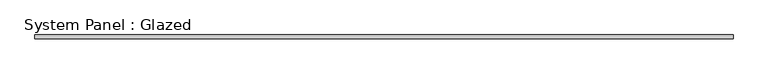
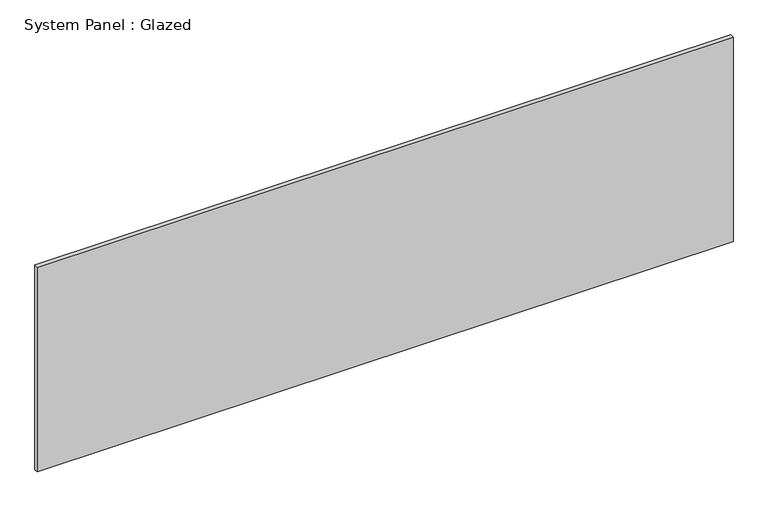
"""IFC4 building model written with IfcOpenShell, lengths in millimetres: plate geometry, System Panel : Glazed."""

from ifc_helpers import new_model, si_unit, origin, origin_with_axes, place, context, project, spatial, polyline, outline, extrude, source, transform, mapped, element, save


def system_panel_glazed_0656cd8c(model_context):
    return source(origin(), model_context, "Body", "SweptSolid", [
        extrude(outline(polyline([(2349.5, 19.05), (-2349.5, 19.05), (-2349.5, 44.45), (2349.5, 44.45), (2349.5, 19.05)])), origin_with_axes(), (0.0, 0.0, 1.0), 1460.5),
    ])


if __name__ == "__main__":
    model = new_model("IFC4")
    model_context = context("Model", 3, world=origin())
    ifc_project = project(units=[si_unit("LENGTHUNIT", "METRE", prefix="MILLI")], contexts=[model_context])
    site = spatial("IfcSite", under=ifc_project)
    building = spatial("IfcBuilding", under=site)
    placement = place(None, origin())
    system_panel_glazed_shape = system_panel_glazed_0656cd8c(model_context)
    element("IfcPlate", 1, ObjectType="System Panel : Glazed", at=placement, inside=building, context=model_context, shape_type="MappedRepresentation", body=[
        mapped(system_panel_glazed_shape, transform((0.0, 0.0, 0.0), x_axis=(1.0, 0.0, 0.0), y_axis=(0.0, 1.0, 0.0), z_axis=(0.0, 0.0, 1.0))),
    ])
    save(model, "model.ifc")

# Revit data of these elements
# Type "System Panel : Glazed"
#   Construction Type Id = "GSP4R"
#   Analytic Construction = "1/8 in Pilkington single glazing"
#   Visual Light Transmittance = 0.9
#   Solar Heat Gain Coefficient = 0.86
#   Heat Transfer Coefficient (U) = 1.18115 BTU/(h·ft²·°F)
# Element 1 (IfcPlate, "System Panel : Glazed")
#   Materials on its faces: "Glass"
# Materials
#   "Glass": class "Glass", colour RGB 0 128 192, transparency 0.75, Description = "Soda Lime Glass", Cost = 0
